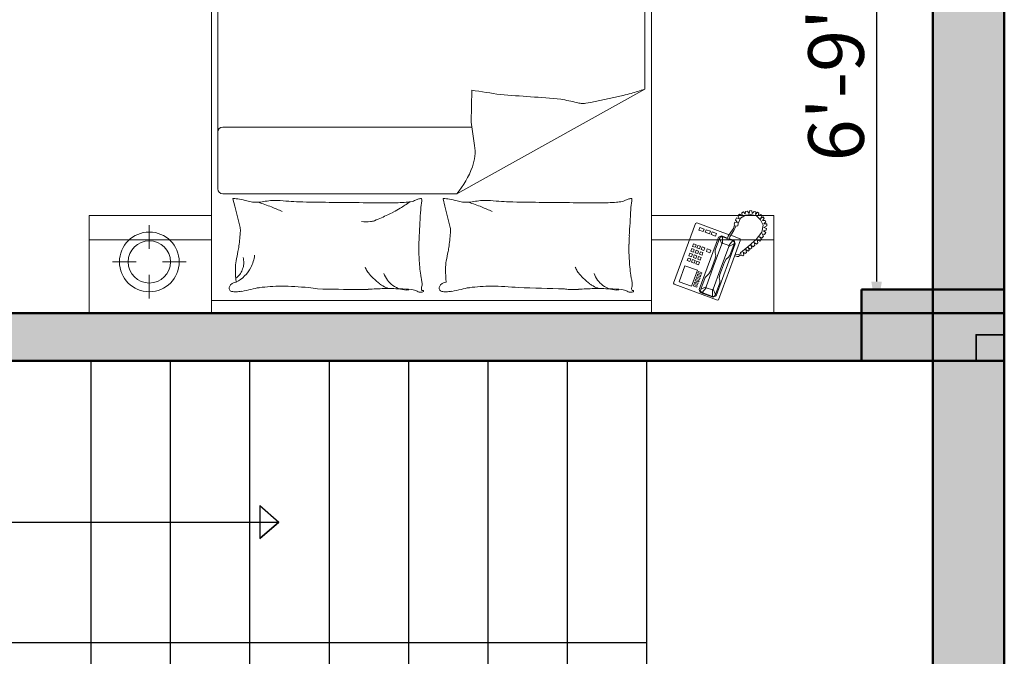
# Model space of a CAD drawing. Units: inches. Extents: x -7 to 1228, y -146 to 1091.
# Tile 83 of 88: x 1003 to 1127, y 531 to 611. Entities that reach past the tile are written whole.
import ezdxf

# ---------------------------------------------------------------- set-up
doc = ezdxf.new("R2010")
doc.units = ezdxf.units.IN
for name, color, linetype, lineweight in [('A-ANNO-DIMS', 2, 'Continuous', 18), ('A-COLS', 6, 'Continuous', 35), ('A-FLOR-STRS', 1, 'Continuous', 25), ('A-FURN', 8, 'Continuous', 18), ('A-WALL', 7, 'Continuous', 50), ('A-WALL-PATT', 251, 'Continuous', 13)]:
    doc.layers.add(name, color=color, linetype=linetype, lineweight=lineweight)
doc.styles.add('DIM_FONT', font='SIMPLEX.shx', dxfattribs={"width": 0.8})
doc.styles.get("Standard").update_dxf_attribs({"font": 'arial.ttf'})
doc.dimstyles.new('ISO-25', dxfattribs={"dimtxt": 7, "dimasz": 4, "dimexe": 1.25, "dimexo": 0.625, "dimtad": 1, "dimdec": 1, "dimlunit": 3, "dimtxsty": 'Standard', "dimcen": 2.5, "dimadec": 0, "dimazin": 0, "dimtfac": 1, "dimtdec": 1, "dimtmove": 1, "dimatfit": 3, "dimfxl": 1, "dimarcsym": 0})

# ---------------------------------------------------------------- blocks, each defined once
blk = doc.blocks.new('A$C4F634EDD')
for p, q in [((0, 2.6295), (0, 2.2295)), ((0.5, 2.6295), (0, 2.6295)), ((0.5, 2.6295), (2.3, 2.6295)), ((0.5, 0.5295), (0.5, 2.6295)), ((0.5, 2.2295), (0.5, 2.6295)), ((2.3, 2.6295), (2.3, 0.5295)), ((2.3, 2.6295), (2.8, 2.6295)), ((2.3, 2.2295), (2.3, 2.6295)), ((2.8, 2.6295), (2.8, 2.2295)), ((0.2457, 2.5697), (0.2457, 2.4733)), ((0.5, 2.5771), (2.3, 2.5771)), ((2.392, 2.5115), (2.5692, 2.5765)), ((2.4946, 2.5331), (2.4985, 2.5445)), ((2.4985, 2.5445), (2.5516, 2.564)), ((2.5062, 2.5454), (2.5004, 2.5392)), ((2.5004, 2.5392), (2.5013, 2.5315)), ((2.5062, 2.5454), (2.5487, 2.561)), ((2.5235, 2.5256), (2.5062, 2.5454)), ((2.5483, 2.5347), (2.5487, 2.561)), ((2.5487, 2.561), (2.5571, 2.56)), ((2.5615, 2.5536), (2.5514, 2.5318)), ((2.5516, 2.564), (2.5637, 2.5584)), ((2.5571, 2.56), (2.5615, 2.5536)), ((2.5615, 2.5536), (2.5791, 2.5058)), ((2.5637, 2.5584), (2.6418, 2.3458)), ((2.5692, 2.5765), (2.574, 2.5743)), ((2.574, 2.5743), (2.6638, 2.3298)), ((2.3898, 2.5066), (2.392, 2.5115)), ((2.4795, 2.2621), (2.3898, 2.5066)), ((2.412, 2.5007), (2.4634, 2.5196)), ((2.4361, 2.4352), (2.412, 2.5007)), ((2.4634, 2.5196), (2.4875, 2.454)), ((2.4842, 2.5232), (2.47, 2.518)), ((2.47, 2.518), (2.472, 2.5127)), ((2.472, 2.5127), (2.4862, 2.5179)), ((2.4881, 2.5126), (2.4739, 2.5074)), ((2.4739, 2.5074), (2.4759, 2.502)), ((2.4759, 2.502), (2.4901, 2.5073)), ((2.492, 2.5019), (2.4778, 2.4967)), ((2.4778, 2.4967), (2.4798, 2.4914)), ((2.4862, 2.5179), (2.4842, 2.5232)), ((2.4901, 2.5073), (2.4881, 2.5126)), ((2.494, 2.4966), (2.492, 2.5019)), ((2.5734, 2.3187), (2.4946, 2.5331)), ((2.5013, 2.5315), (2.5188, 2.4836)), ((2.5013, 2.5315), (2.5231, 2.5214)), ((2.5231, 2.5214), (2.5235, 2.5256)), ((2.5523, 2.4417), (2.5231, 2.5214)), ((2.5483, 2.5347), (2.5235, 2.5256)), ((2.5514, 2.5318), (2.5483, 2.5347)), ((2.5807, 2.4521), (2.5514, 2.5318)), ((2.5791, 2.5058), (2.5788, 2.4956)), ((2.4798, 2.4914), (2.494, 2.4966)), ((2.4959, 2.4913), (2.4817, 2.4861)), ((2.4817, 2.4861), (2.4837, 2.4808)), ((2.4837, 2.4808), (2.4979, 2.486)), ((2.4998, 2.4807), (2.4856, 2.4755)), ((2.4856, 2.4755), (2.4876, 2.4702)), ((2.4876, 2.4702), (2.5018, 2.4754)), ((2.5037, 2.47), (2.4895, 2.4648)), ((2.4895, 2.4648), (2.4915, 2.4595)), ((2.4915, 2.4595), (2.5057, 2.4647)), ((2.4979, 2.486), (2.4959, 2.4913)), ((2.5018, 2.4754), (2.4998, 2.4807)), ((2.5057, 2.4647), (2.5037, 2.47)), ((2.5188, 2.4836), (2.5256, 2.4761)), ((2.5256, 2.4761), (2.5342, 2.4692)), ((2.5342, 2.4692), (2.5405, 2.4574)), ((2.5405, 2.4574), (2.547, 2.4397)), ((2.5788, 2.4956), (2.5767, 2.4848)), ((2.5767, 2.4848), (2.5795, 2.4717)), ((2.5795, 2.4717), (2.586, 2.454)), ((0.0957, 2.4197), (0.192, 2.4197)), ((0.2994, 2.4197), (0.3957, 2.4197)), ((2.4875, 2.454), (2.4361, 2.4352)), ((2.4457, 2.4146), (2.4563, 2.4185)), ((2.4563, 2.4185), (2.4602, 2.4078)), ((2.4634, 2.4211), (2.474, 2.425)), ((2.4673, 2.4104), (2.4634, 2.4211)), ((2.474, 2.425), (2.4779, 2.4143)), ((2.4811, 2.4276), (2.4917, 2.4315)), ((2.485, 2.4169), (2.4811, 2.4276)), ((2.4956, 2.4208), (2.485, 2.4169)), ((2.4917, 2.4315), (2.4956, 2.4208)), ((2.5594, 2.4061), (2.547, 2.4397)), ((2.5523, 2.4417), (2.5875, 2.346)), ((2.5807, 2.4521), (2.6158, 2.3564)), ((2.5984, 2.4204), (2.586, 2.454)), ((2.6047, 2.4086), (2.5984, 2.4204)), ((2.4496, 2.4039), (2.4457, 2.4146)), ((2.4602, 2.4078), (2.4496, 2.4039)), ((2.4528, 2.3951), (2.4635, 2.399)), ((2.4567, 2.3844), (2.4528, 2.3951)), ((2.4674, 2.3883), (2.4567, 2.3844)), ((2.46, 2.3756), (2.4706, 2.3795)), ((2.4635, 2.399), (2.4674, 2.3883)), ((2.4779, 2.4143), (2.4673, 2.4104)), ((2.4706, 2.4016), (2.4812, 2.4055)), ((2.4745, 2.3909), (2.4706, 2.4016)), ((2.4706, 2.3795), (2.4745, 2.3689)), ((2.4851, 2.3949), (2.4745, 2.3909)), ((2.4777, 2.3821), (2.4883, 2.386)), ((2.4816, 2.3715), (2.4777, 2.3821)), ((2.4812, 2.4055), (2.4851, 2.3949)), ((2.4883, 2.4081), (2.4989, 2.412)), ((2.4922, 2.3975), (2.4883, 2.4081)), ((2.4883, 2.386), (2.4922, 2.3754)), ((2.5028, 2.4014), (2.4922, 2.3975)), ((2.4954, 2.3886), (2.5061, 2.3925)), ((2.4993, 2.378), (2.4954, 2.3886)), ((2.4989, 2.412), (2.5028, 2.4014)), ((2.51, 2.3819), (2.4993, 2.378)), ((2.5061, 2.3925), (2.51, 2.3819)), ((2.5238, 2.3769), (2.538, 2.3821)), ((2.5277, 2.3663), (2.5238, 2.3769)), ((2.538, 2.3821), (2.5419, 2.3715)), ((2.5622, 2.393), (2.5594, 2.4061)), ((2.5598, 2.372), (2.5601, 2.3822)), ((2.5601, 2.3822), (2.5622, 2.393)), ((2.6133, 2.4017), (2.6047, 2.4086)), ((2.6201, 2.3941), (2.6133, 2.4017)), ((2.6376, 2.3463), (2.6201, 2.3941)), ((2.6499, 2.3979), (2.6397, 2.3953)), ((2.6417, 2.39), (2.6488, 2.391)), ((2.6488, 2.391), (2.6538, 2.3895)), ((2.6551, 2.397), (2.6499, 2.3979)), ((2.6538, 2.3895), (2.6596, 2.388)), ((2.6627, 2.392), (2.6551, 2.397)), ((2.6596, 2.388), (2.6626, 2.3867)), ((2.6626, 2.3867), (2.6662, 2.388)), ((2.6692, 2.394), (2.6627, 2.392)), ((2.6662, 2.388), (2.6632, 2.3828)), ((2.6632, 2.3828), (2.6736, 2.3744)), ((2.6736, 2.3944), (2.6692, 2.394)), ((2.6765, 2.391), (2.6736, 2.3944)), ((2.6742, 2.3795), (2.6765, 2.391)), ((2.6824, 2.3858), (2.6742, 2.3795)), ((2.6873, 2.3815), (2.6824, 2.3858)), ((2.6853, 2.369), (2.6873, 2.3815)), ((2.6946, 2.376), (2.6853, 2.369)), ((2.6995, 2.3713), (2.6946, 2.376)), ((0.2457, 2.366), (0.2457, 2.2697)), ((2.4639, 2.365), (2.46, 2.3756)), ((2.4745, 2.3689), (2.4639, 2.365)), ((2.4672, 2.3561), (2.4778, 2.36)), ((2.4711, 2.3455), (2.4672, 2.3561)), ((2.4817, 2.3494), (2.4711, 2.3455)), ((2.4778, 2.36), (2.4817, 2.3494)), ((2.4922, 2.3754), (2.4816, 2.3715)), ((2.4849, 2.3626), (2.4955, 2.3665)), ((2.4888, 2.352), (2.4849, 2.3626)), ((2.4994, 2.3559), (2.4888, 2.352)), ((2.4955, 2.3665), (2.4994, 2.3559)), ((2.5026, 2.3691), (2.5132, 2.373)), ((2.5065, 2.3585), (2.5026, 2.3691)), ((2.5171, 2.3624), (2.5065, 2.3585)), ((2.5132, 2.373), (2.5171, 2.3624)), ((2.5419, 2.3715), (2.5277, 2.3663)), ((2.5774, 2.3242), (2.5598, 2.372)), ((2.5774, 2.3242), (2.5875, 2.346)), ((2.5875, 2.346), (2.5905, 2.3431)), ((2.5905, 2.3431), (2.5901, 2.3168)), ((2.6154, 2.3522), (2.5905, 2.3431)), ((2.6158, 2.3564), (2.6154, 2.3522)), ((2.6154, 2.3522), (2.6327, 2.3324)), ((2.6376, 2.3463), (2.6158, 2.3564)), ((2.6327, 2.3324), (2.6385, 2.3386)), ((2.6418, 2.3458), (2.6369, 2.332)), ((2.6385, 2.3386), (2.6376, 2.3463)), ((2.6736, 2.3744), (2.6922, 2.3593)), ((2.6922, 2.3593), (2.7051, 2.3473)), ((2.695, 2.3603), (2.6995, 2.3713)), ((2.7031, 2.3682), (2.695, 2.3603)), ((2.7096, 2.3616), (2.7031, 2.3682)), ((2.7051, 2.3473), (2.7079, 2.3475)), ((2.7062, 2.351), (2.7096, 2.3616)), ((2.7147, 2.3578), (2.7062, 2.351)), ((2.7079, 2.3475), (2.7079, 2.3443)), ((2.7079, 2.3443), (2.727, 2.3277)), ((2.7214, 2.3517), (2.7147, 2.3578)), ((2.7196, 2.34), (2.7214, 2.3517)), ((2.7286, 2.3466), (2.7196, 2.34)), ((2.7346, 2.3423), (2.7286, 2.3466)), ((2.732, 2.3295), (2.7346, 2.3423)), ((0, 2.3301), (0.5, 2.3301)), ((2.8, 2.3301), (2.3, 2.3301)), ((2.6172, 2.3086), (2.4844, 2.2599)), ((2.5114, 2.2959), (2.4936, 2.2894)), ((2.5153, 2.2853), (2.5114, 2.2959)), ((2.5362, 2.305), (2.5185, 2.2985)), ((2.5185, 2.2985), (2.5224, 2.2879)), ((2.5401, 2.2944), (2.5362, 2.305)), ((2.561, 2.3141), (2.5433, 2.3076)), ((2.5433, 2.3076), (2.5472, 2.297)), ((2.5472, 2.297), (2.5649, 2.3035)), ((2.5649, 2.3035), (2.561, 2.3141)), ((2.5855, 2.3131), (2.5734, 2.3187)), ((2.5818, 2.3178), (2.5774, 2.3242)), ((2.5901, 2.3168), (2.5818, 2.3178)), ((2.6104, 2.3222), (2.5855, 2.3131)), ((2.5901, 2.3168), (2.6097, 2.324)), ((2.613, 2.3312), (2.6077, 2.3293)), ((2.6077, 2.3293), (2.6135, 2.3141)), ((2.6192, 2.3174), (2.613, 2.3312)), ((2.6135, 2.3141), (2.6244, 2.2977)), ((2.6153, 2.3261), (2.6327, 2.3324)), ((2.6369, 2.332), (2.6161, 2.3243)), ((2.626, 2.3069), (2.6192, 2.3174)), ((2.6616, 2.3249), (2.6234, 2.3109)), ((2.6244, 2.2977), (2.6349, 2.2825)), ((2.6365, 2.2916), (2.626, 2.3069)), ((2.6638, 2.3298), (2.6616, 2.3249)), ((2.727, 2.3277), (2.7512, 2.2983)), ((2.7423, 2.3345), (2.732, 2.3295)), ((2.7406, 2.3172), (2.7495, 2.325)), ((2.7519, 2.3218), (2.7406, 2.3172)), ((2.7495, 2.325), (2.7423, 2.3345)), ((2.7512, 2.2983), (2.756, 2.2695)), ((2.7575, 2.3144), (2.7519, 2.3218)), ((2.7526, 2.3045), (2.7575, 2.3144)), ((2.7622, 2.308), (2.7526, 2.3045)), ((2.7574, 2.2924), (2.7673, 2.2997)), ((2.7673, 2.2997), (2.7622, 2.308)), ((0.5953, 2.1912), (0.616, 2.2738)), ((1.4546, 2.1912), (1.4752, 2.2738)), ((2.4844, 2.2599), (2.4795, 2.2621)), ((2.4936, 2.2894), (2.4976, 2.2788)), ((2.4976, 2.2788), (2.5153, 2.2853)), ((2.5224, 2.2879), (2.5401, 2.2944)), ((2.6349, 2.2825), (2.638, 2.273)), ((2.6407, 2.2834), (2.6365, 2.2916)), ((2.6399, 2.2712), (2.6374, 2.2659)), ((2.6374, 2.2659), (2.6398, 2.257)), ((2.638, 2.273), (2.6399, 2.2712)), ((2.6398, 2.257), (2.6509, 2.259)), ((2.6438, 2.2739), (2.6407, 2.2834)), ((2.6509, 2.259), (2.6431, 2.2492)), ((2.6519, 2.2716), (2.6438, 2.2739)), ((2.6535, 2.2628), (2.6519, 2.2716)), ((2.6636, 2.2409), (2.6535, 2.2628)), ((2.756, 2.2695), (2.7459, 2.2483)), ((2.7687, 2.2905), (2.7574, 2.2924)), ((2.7587, 2.279), (2.7699, 2.2828)), ((2.7708, 2.2725), (2.7587, 2.279)), ((2.759, 2.2637), (2.7706, 2.2643)), ((2.7676, 2.2559), (2.759, 2.2637)), ((2.7645, 2.2498), (2.7676, 2.2559)), ((2.7699, 2.2828), (2.7687, 2.2905)), ((2.7706, 2.2643), (2.7708, 2.2725)), ((0, 2.2295), (0.5, 2.2295)), ((2.8, 2.2295), (2.3, 2.2295)), ((2.6431, 2.2492), (2.6473, 2.2398)), ((2.6473, 2.2398), (2.6592, 2.2429)), ((2.6592, 2.2429), (2.6521, 2.2314)), ((2.6521, 2.2314), (2.6598, 2.2248)), ((2.6598, 2.2248), (2.6697, 2.2309)), ((2.6836, 2.2287), (2.6636, 2.2409)), ((2.6697, 2.2309), (2.6684, 2.219)), ((2.6684, 2.219), (2.6761, 2.2145)), ((2.6761, 2.2145), (2.6821, 2.2237)), ((2.6821, 2.2237), (2.6843, 2.2135)), ((2.7063, 2.2256), (2.6836, 2.2287)), ((2.6927, 2.2117), (2.6986, 2.222)), ((2.6986, 2.222), (2.7019, 2.2098)), ((2.7284, 2.2317), (2.7063, 2.2256)), ((2.7102, 2.2104), (2.7113, 2.2218)), ((2.7113, 2.2218), (2.7192, 2.2137)), ((2.7192, 2.2137), (2.7255, 2.2152)), ((2.7255, 2.2152), (2.7242, 2.2265)), ((2.7242, 2.2265), (2.7324, 2.2165)), ((2.7459, 2.2483), (2.7284, 2.2317)), ((2.7324, 2.2165), (2.7386, 2.2208)), ((2.7386, 2.2208), (2.7354, 2.2306)), ((2.7354, 2.2306), (2.7462, 2.2264)), ((2.7509, 2.2314), (2.7459, 2.2418)), ((2.7459, 2.2418), (2.7568, 2.2352)), ((2.7462, 2.2264), (2.7509, 2.2314)), ((2.7529, 2.2505), (2.7645, 2.2498)), ((2.7607, 2.2424), (2.7529, 2.2505)), ((2.7568, 2.2352), (2.7607, 2.2424)), ((0.5878, 2.1612), (0.5953, 2.1912)), ((1.4471, 2.1612), (1.4546, 2.1912)), ((2.6843, 2.2135), (2.6927, 2.2117)), ((2.7019, 2.2098), (2.7102, 2.2104)), ((1.5035, 2.141), (0.5458, 2.141)), ((1.5035, 2.141), (2.2716, 1.7136)), ((0.5258, 2.121), (0.5258, 0.5617)), ((1.576, 1.9433), (1.5624, 1.8479)), ((0.5458, 1.8684), (1.5653, 1.8684)), ((1.5624, 1.8479), (1.5641, 1.7178)), ((2.2716, 0.5617), (2.2716, 1.7136))]:
    blk.add_line(p, q)
for radius in [0.1222, 0.0865]:
    blk.add_circle((0.2457, 2.4197), radius)
for centre, radius, start, end in [((0.5848, 2.5274), 0.0131, 101.2724, 206.5805), ((0.5999, 2.4516), 0.0904, 90, 101.2724), ((0.5999, 2.3808), 0.1611, 81.5628, 90), ((0.5788, 2.2388), 0.3048, 74.256, 81.5628), ((1.3132, 2.5864), 0.0539, 275.2592, 300.6513), ((1.3554, 2.5152), 0.0289, 85.6975, 120.6513), ((1.3556, 2.519), 0.0251, 68.2117, 85.6975), ((1.3634, 2.533), 0.00428, 78.1069, 158.0096), ((1.3647, 2.5395), 0.00232, 258.1069, 19.564), ((1.3637, 2.5391), 0.00342, 19.564, 68.2117), ((1.444, 2.5274), 0.0131, 101.2724, 206.5805), ((1.4591, 2.4516), 0.0904, 90, 101.2724), ((1.4591, 2.3808), 0.1611, 81.5628, 90), ((1.438, 2.2388), 0.3048, 74.256, 81.5628), ((2.1724, 2.5864), 0.0539, 275.2592, 300.6513), ((2.2146, 2.5152), 0.0289, 85.6975, 120.6513), ((2.2149, 2.519), 0.0251, 68.2117, 85.6975), ((2.2226, 2.533), 0.00428, 78.1069, 158.0096), ((2.224, 2.5395), 0.00232, 258.1069, 19.564), ((2.2229, 2.5391), 0.00342, 19.564, 68.2117), ((0.6036, 2.5368), 0.0342, 206.5805, 265.5998), ((1.0898, 2.4496), 0.4918, 173.7676, 180), ((0.5368, 2.3783), 0.1399, 45.0976, 62.7964), ((0.7272, 2.7653), 0.2422, 254.256, 262.4531), ((0.7851, 3.2019), 0.6827, 262.4531, 270), ((0.7851, 3.5682), 1.049, 270, 276.0867), ((0.8402, 3.0514), 0.5293, 276.0867, 280.1899), ((1.1602, -8.1346), 10.6675, 90.30153, 91.21582), ((1.1169, 2.2433), 0.2897, 85.1982, 92.5386), ((1.2142, 3.4021), 0.8732, 265.1982, 269.4243), ((1.4317, 2.2032), 0.3916, 128.3886, 133.8115), ((1.2362, 2.45), 0.0768, 117.2396, 128.3886), ((1.3082, 2.3102), 0.234, 110.8603, 117.2396), ((1.2204, 4.0232), 1.4943, 269.4243, 271.9079), ((1.2995, 2.4357), 0.0992, 126.0864, 143.8234), ((1.2995, 2.4357), 0.0992, 105.9352, 126.0864), ((1.2429, 3.3501), 0.8208, 271.9079, 275.2592), ((1.2995, 2.4357), 0.0992, 85.7841, 105.9352), ((1.3739, 2.5288), 0.0156, 158.0096, 201.421), ((1.1177, 2.5413), 0.246, 347.8905, 351.8665), ((1.3288, 2.5111), 0.0328, 351.8665, 21.421), ((1.4628, 2.5368), 0.0342, 206.5805, 265.5998), ((1.949, 2.4496), 0.4918, 173.7676, 180), ((1.5865, 2.7653), 0.2422, 254.256, 262.4531), ((1.6443, 3.2019), 0.6827, 262.4531, 270), ((1.6443, 3.5682), 1.049, 270, 276.0867), ((1.4785, 15.4878), 12.9656, 271.22425, 272.05324), ((1.97, 2.3805), 0.1524, 92.5386, 100.1899), ((1.9761, 2.2433), 0.2897, 85.1982, 92.5386), ((2.0734, 3.4021), 0.8732, 265.1982, 269.4243), ((2.291, 2.2032), 0.3916, 128.3886, 133.8115), ((2.0954, 2.45), 0.0768, 117.2396, 128.3886), ((2.1674, 2.3102), 0.234, 110.8603, 117.2396), ((2.0797, 4.0232), 1.4943, 269.4243, 271.9079), ((2.1588, 2.4357), 0.0992, 126.0864, 143.8234), ((2.1588, 2.4357), 0.0992, 105.9352, 126.0864), ((2.1021, 3.3501), 0.8208, 271.9079, 275.2592), ((2.1588, 2.4357), 0.0992, 85.7841, 105.9352), ((2.2331, 2.5288), 0.0156, 158.0096, 201.421), ((1.977, 2.5413), 0.246, 347.8905, 351.8665), ((2.1881, 2.5111), 0.0328, 351.8665, 21.421), ((0.5462, 2.4142), 0.0899, 41.4429, 53.7359), ((0.5741, 2.4389), 0.0526, 25.3551, 41.4429), ((0.4851, 2.3967), 0.1511, 21.8149, 25.3551), ((0.5368, 2.3783), 0.1399, 27.3988, 45.0976), ((1.3127, 2.3625), 0.2002, 151.6832, 156.9972), ((1.1799, 2.4341), 0.0493, 140.9651, 151.6832), ((1.3165, 2.3233), 0.2252, 133.8115, 140.9651), ((1.2995, 2.4357), 0.0992, 143.8234, 161.5603), ((2.2605, 2.3525), 0.9131, 172.3191, 176.6313), ((1.5522, 2.448), 0.1983, 167.8905, 172.3191), ((2.1719, 2.3625), 0.2002, 151.6832, 156.9972), ((2.0391, 2.4341), 0.0493, 140.9651, 151.6832), ((2.1757, 2.3233), 0.2252, 133.8115, 140.9651), ((2.1588, 2.4357), 0.0992, 143.8234, 161.5603), ((3.1198, 2.3525), 0.9131, 172.3191, 176.6313), ((2.4114, 2.448), 0.1983, 167.8905, 172.3191), ((0.8019, 2.4496), 0.204, 180, 189.6844), ((0.4345, 2.3765), 0.2056, 18.7799, 21.8149), ((0.576, 2.4246), 0.0562, 0, 18.7799), ((0.5406, 2.4246), 0.0915, 345.3149, 0), ((0.5368, 2.3783), 0.1399, 16.515, 27.3988), ((0.5368, 2.3783), 0.1399, 5.6311, 16.515), ((1.6611, 2.4496), 0.204, 180, 189.6844), ((1.4703, 2.5637), 0.882, 189.6844, 192.1984), ((0.2982, 2.3103), 0.3171, 8.0051, 12.1984), ((2.0266, 2.3663), 0.6787, 176.6313, 181.6331), ((2.3295, 2.5637), 0.882, 189.6844, 192.1984), ((1.1575, 2.3103), 0.3171, 8.0051, 12.1984), ((2.8858, 2.3663), 0.6787, 176.6313, 181.6331), ((-0.0401, 2.2627), 0.6588, 2.6649, 8.0051), ((2.7128, 2.3859), 1.3652, 181.6331, 183.055), ((0.8191, 2.2627), 0.6588, 2.6649, 8.0051), ((3.5721, 2.3859), 1.3652, 181.6331, 183.055), ((14.9657, 3.0398), 13.6356, 183.05496, 183.50486), ((15.8249, 3.0398), 13.6356, 183.05496, 183.50486), ((0.5503, 2.2902), 0.0677, 345.9548, 2.6649), ((1.1303, 1.9835), 0.2721, 85.9172, 93.5552), ((1.4096, 2.2902), 0.0677, 345.9548, 2.6649), ((1.1455, 2.197), 0.058, 69.3257, 85.9172), ((0.9871, 1.7772), 0.5066, 65.6735, 69.3257), ((0.6058, 0.9338), 1.4323, 63.5015, 65.6735), ((1.1054, 1.9358), 0.3126, 57.865, 63.5015), ((0.6807, 2.0561), 0.1197, 96.4341, 107.3864), ((0.6836, 2.0301), 0.1459, 78.4414, 96.4341), ((0.473, 2.8815), 0.7387, 287.1982, 289.428), ((0.473, 2.8815), 0.7387, 289.428, 291.6577), ((0.473, 2.8815), 0.7387, 291.6577, 293.4844), ((0.473, 2.8815), 0.7387, 293.4844, 295.3111), ((1.2501, -19.8405), 22.0183, 90.37908, 91.01965), ((1.2012, -3.5404), 5.7185, 89.7135, 90.9704), ((1.224, 1.0141), 1.164, 86.426, 89.7135), ((0.8841, 1.5835), 0.7286, 54.1737, 57.865), ((1.2875, 2.0302), 0.1459, 77.131, 86.426), ((1.6762, 2.2258), 0.3212, 183.5049, 189.9984), ((1.5399, 2.0561), 0.1197, 96.4341, 107.3864), ((1.5429, 2.0301), 0.1459, 78.4414, 96.4341), ((1.3322, 2.8815), 0.7387, 287.1982, 289.428), ((1.3322, 2.8815), 0.7387, 289.428, 291.6577), ((1.3322, 2.8815), 0.7387, 291.6577, 293.4844), ((1.3322, 2.8815), 0.7387, 293.4844, 295.3111), ((2.1093, -19.8405), 22.0183, 90.37908, 91.01965), ((2.0605, -3.5404), 5.7185, 89.7135, 90.9704), ((2.0833, 1.0141), 1.164, 86.426, 89.7135), ((2.1467, 2.0302), 0.1459, 77.131, 86.426), ((2.5355, 2.2258), 0.3212, 183.5049, 189.9984), ((0.5458, 2.121), 0.02, 90, 180), ((0.5887, 2.1609), 0.000917, 165.9551, 274.0829), ((0.5695, 2.4301), 0.2708, 274.0829, 279.4841), ((0.5763, 2.3896), 0.2297, 279.4841, 287.3864), ((0.759, 2.3985), 0.2301, 258.4414, 272.7491), ((0.7026, 3.5718), 1.4048, 272.7491, 274.6176), ((0.9136, 0.9591), 1.2165, 92.6096, 94.6176), ((1.3099, 2.1283), 0.0453, 62.7159, 77.131), ((1.3658, 2.2367), 0.0767, 242.7159, 253.7788), ((1.3688, 2.247), 0.0875, 253.7788, 262.8796), ((1.3581, 2.1615), 0.00132, 262.8796, 343.3022), ((1.3409, 2.1667), 0.0193, 343.3022, 9.9984), ((1.448, 2.1609), 0.000917, 165.9551, 274.0829), ((1.4288, 2.4301), 0.2708, 274.0829, 279.4841), ((1.4355, 2.3896), 0.2297, 279.4841, 287.3864), ((1.2147, 1.9017), 0.3751, 20.1488, 39.6445), ((1.6182, 2.3985), 0.2301, 258.4414, 272.7491), ((1.5619, 3.5718), 1.4048, 272.7491, 274.6176), ((1.7729, 0.9591), 1.2165, 92.6096, 94.6176), ((2.1691, 2.1283), 0.0453, 62.7159, 77.131), ((2.2251, 2.2367), 0.0767, 242.7159, 253.7788), ((2.2281, 2.247), 0.0875, 253.7788, 262.8796), ((2.2174, 2.1615), 0.00132, 262.8796, 343.3022), ((2.2001, 2.1667), 0.0193, 343.3022, 9.9984), ((1.3977, 1.9688), 0.1801, 351.8644, 20.1488), ((0.5458, 1.8884), 0.02, 180, 270), ((2.0195, 1.7137), 0.0581, 79.2724, 97.7304), ((1.0582, 5.4638), 3.7801, 277.692, 279.495), ((0.6102, 18.0525), 16.3521, 273.75703, 274.62393), ((1.4194, 4.2174), 2.5158, 281.6741, 283.1904), ((2.0378, 1.5789), 0.1942, 97.7304, 103.1904), ((1.2737, -2.2227), 4.0646, 77.0745, 79.2724), ((2.0359, 1.0981), 0.6574, 74.0648, 77.0745), ((1.7125, -0.0344), 1.8351, 72.2636, 74.0648)]:
    blk.add_arc(centre, radius, start, end)
at = {"style": 'DIM_FONT', "width": 0.8, "flags": 9}
for tag, p in [('YSIZE', (0.5, 2.6295)), ('XSIZE', (0.5, 2.6295)), ('XSIZE', (2.2985, 2.6295)), ('YSIZE', (2.2985, 2.6295))]:
    blk.add_attdef(tag, p, '', height=0.0005, dxfattribs=at)
blk = doc.blocks.new('*D27')
at = {"layer": 'A-ANNO-DIMS', "color": 0, "lineweight": -2, "transparency": 16777216}
for p, q in [((1098.61, 654.97), (1112.17, 654.97)), ((1110.92, 650.97), (1110.92, 577.98)), ((1098.61, 573.98), (1112.17, 573.98))]:
    blk.add_line(p, q, dxfattribs=at)
at = {"layer": 'A-ANNO-DIMS', "color": 0, "transparency": 16777216}
for points in [[(1110.25, 650.97), (1111.58, 650.97), (1110.92, 654.97)], [(1110.25, 577.98), (1111.58, 577.98), (1110.92, 573.98)]]:
    blk.add_solid(points, dxfattribs=at)
at = {"layer": 'Defpoints', "color": 0, "transparency": 16777216}
for p in [(1097.98, 654.97), (1097.98, 573.98), (1110.92, 573.98)]:
    blk.add_point(p, dxfattribs=at)
at = {"layer": 'A-ANNO-DIMS', "color": 0, "transparency": 16777216, "insert": (1106.72, 614.48), "char_height": 7, "attachment_point": 5, "rotation": 90}
blk.add_mtext('6\'-9" TYP.', dxfattribs=at)

msp = doc.modelspace()

# ---------------------------------------------------------------- hatches: boundary and pattern name
at = {"layer": 'A-COLS'}
h = msp.add_hatch(color=256, dxfattribs=at)
h.dxf.hatch_style = 1
h.paths.add_polyline_path([(1123.45, 568), (1123.45, 571.29), (1127, 571.29), (1127, 577), (1109, 577), (1109, 568)])
h = msp.add_hatch(color=256, dxfattribs=at)
h.dxf.hatch_style = 1
h.paths.add_polyline_path([(1123.45, 568), (1127, 568), (1127, 571.29), (1123.45, 571.29)])
at = {"layer": 'A-WALL-PATT'}
h = msp.add_hatch(color=256, dxfattribs=at)
h.dxf.hatch_style = 1
h.paths.add_polyline_path([(69, 568), (60, 568), (60, 493), (63.29, 493), (69, 493)])
h.paths.add_polyline_path([(69, 662.41), (60, 662.41), (60, 586), (69, 586)], flags=17)
h.paths.add_polyline_path([(69, 723), (184, 723), (184, 734), (179, 734), (179, 728), (69, 728), (69, 741.62), (60, 741.62), (60, 698.41), (69, 698.41)], flags=17)
h.paths.add_polyline_path([(69, 782), (231, 782), (231, 728), (231, 723), (231, 586), (236, 586), (236, 787), (69, 787), (69, 800.13), (60, 800.13), (60, 765.62), (69, 765.62)])
h.paths.add_polyline_path([(184, 842), (189, 842), (189, 848), (173, 848), (173, 842), (179, 842), (179, 787), (184, 787)])
h.paths.add_polyline_path([(118.22, 69), (69, 69), (69, 60), (118.22, 60)])
h.paths.add_polyline_path([(227, 69), (154.22, 69), (154.22, 60), (227, 60)])
h.paths.add_polyline_path([(236, 60), (232.71, 60), (227, 60), (227, 36), (236, 36)])
h.paths.add_polyline_path([(389, 60), (380, 60), (380, 36), (389, 36)])
h.paths.add_polyline_path([(384, 181), (380, 181), (380, 115), (380, 78), (384, 78)])
h.paths.add_polyline_path([(380, 115), (334.55, 115), (334.55, 109), (380, 109)])
h.paths.add_polyline_path([(274.55, 115), (236, 115), (236, 201), (232.71, 201), (231, 201), (231, 78), (236, 78), (236, 109), (274.55, 109)])
h.paths.add_polyline_path([(69, 123), (60, 123), (60, 78), (69, 78)])
h.paths.add_polyline_path([(69, 201), (60, 201), (60, 159), (69, 159)])
h.paths.add_polyline_path([(143, 219), (69, 219), (69, 213), (143, 213)], flags=17)
h.paths.add_polyline_path([(189, 219), (184, 219), (184, 274), (231, 274), (231, 219), (236, 219), (236, 279), (184, 279), (184, 297), (179, 297), (179, 279), (69, 279), (69, 290.91), (60, 290.91), (60, 262.18), (69, 262.18), (69, 274), (179, 274), (179, 219), (173, 219), (173, 213), (189, 213)])
h.paths.add_polyline_path([(69, 238.18), (60, 238.18), (60, 219), (69, 219)], flags=17)
h.paths.add_polyline_path([(69, 333), (60, 333), (60, 314.91), (69, 314.91), (69, 316.96)])
h.paths.add_polyline_path([(190, 338), (184, 338), (69, 338), (69, 333), (179, 333), (179, 327), (184, 327), (184, 333.02), (190, 333.05)])
h.paths.add_polyline_path([(69, 386.81), (60, 386.81), (60, 351), (69, 351)])
h.paths.add_polyline_path([(69, 475), (60, 475), (60, 422.81), (69, 422.81)])
h.paths.add_polyline_path([(236, 475), (231, 475), (231, 351.24), (236, 351.24)])
h.paths.add_polyline_path([(384, 475), (380, 475), (380, 362), (384, 362)])
h.paths.add_polyline_path([(547, 307), (439, 307), (439, 356), (445, 356), (445, 362), (433, 362), (433, 307), (380, 307), (380, 244), (380, 241), (384, 241), (384, 301), (433, 301), (433, 277), (439, 277), (439, 301), (547, 301)])
h.paths.add_polyline_path([(547, 241), (439, 241), (439, 247), (433, 247), (433, 235), (547, 235)])
h.paths.add_polyline_path([(450, 69), (440.29, 69), (424.89, 69), (389, 69), (389, 60), (450, 60)])
h.paths.add_polyline_path([(547, 69), (486, 69), (486, 60), (547, 60)])
h.paths.add_polyline_path([(556, 148.27), (547, 148.27), (547, 78), (556, 78)])
h.paths.add_polyline_path([(556, 223), (547, 223), (547, 195), (547, 184.27), (556, 184.27)])
h.paths.add_polyline_path([(556, 311.19), (547, 311.19), (547, 273.08), (556, 273.08)])
h.paths.add_polyline_path([(556, 344), (552.71, 344), (547, 344), (547, 335.19), (556, 335.19)])
h.paths.add_polyline_path([(556, 249.08), (547, 249.08), (547, 241), (556, 241)])
h.paths.add_polyline_path([(547, 362), (475, 362), (475, 356), (547, 356)], flags=0)
h.paths.add_polyline_path([(556, 399.62), (547, 399.62), (547, 362), (556, 362)])
h.paths.add_polyline_path([(556, 475), (547, 475), (547, 435.62), (556, 435.62)])
h.paths.add_polyline_path([(547, 493), (389, 493), (389, 487), (547, 487)])
h.paths.add_polyline_path([(380, 493), (278, 493), (278, 487), (380, 487)])
h.paths.add_polyline_path([(227, 493), (69, 493), (69, 487), (227, 487)])
h.paths.add_polyline_path([(643, 122.44), (634, 122.44), (634, 78), (643, 78)])
h.paths.add_polyline_path([(702.5, 69), (692.79, 69), (677.39, 69), (643, 69), (643, 60), (702.5, 60)])
h.paths.add_polyline_path([(798, 69), (738.5, 69), (738.5, 60), (798, 60)])
h.paths.add_polyline_path([(807, 60), (803.71, 60), (798, 60), (798, 36), (807, 36)])
h.paths.add_polyline_path([(807, 109), (846.75, 109), (846.75, 115), (807, 115), (807, 159), (802, 159), (802, 78), (807, 78)])
h.paths.add_polyline_path([(807, 201), (802, 201), (802, 195), (807, 195)])
h.paths.add_polyline_path([(643, 201), (634, 201), (634, 158.44), (643, 158.44)])
h.paths.add_polyline_path([(756, 225), (751, 225), (751, 219), (643, 219), (643, 213), (756, 213)])
h.paths.add_polyline_path([(643, 240.85), (634, 240.85), (634, 219), (643, 219)])
h.paths.add_polyline_path([(643, 274), (643, 288.63), (634, 288.63), (634, 264.85), (643, 264.85)])
h.paths.add_polyline_path([(802, 279), (756, 279), (756, 297), (751, 297), (751, 279), (643, 279), (643, 274), (751, 274), (751, 255), (756, 255), (756, 274), (802, 274)])
h.paths.add_polyline_path([(807, 333), (803.71, 333), (802, 333), (802, 279), (802, 274), (802, 219), (807, 219)])
h.paths.add_polyline_path([(956, 182), (951, 182), (951, 115), (906.75, 115), (906.75, 109), (951, 109), (951, 78), (956, 78)])
h.paths.add_polyline_path([(960, 60), (951, 60), (951, 36), (960, 36)])
h.paths.add_polyline_path([(1021, 69), (1005.78, 69), (960, 69), (960, 60), (1021, 60)])
h.paths.add_polyline_path([(956, 224), (951, 224), (951, 218), (956, 218)])
h.paths.add_polyline_path([(956, 302), (1004, 302), (1004, 278), (1010, 278), (1010, 302), (1118, 302), (1118, 290.81), (1127, 290.81), (1127, 326.97), (1118, 326.97), (1118, 320.97), (1118, 307), (1010, 307), (1010, 356), (1016, 356), (1016, 362), (1004, 362), (1004, 307), (951, 307), (951, 244), (951, 242), (954.29, 242), (956, 242)])
h.paths.add_polyline_path([(643, 333), (634, 333), (634, 312.63), (643, 312.63), (643, 316.96)])
h.paths.add_polyline_path([(756, 338), (643, 338), (643, 333), (751, 333), (751, 327), (756, 327)])
h.paths.add_polyline_path([(643, 388), (634, 388), (634, 351), (643, 351)])
h.paths.add_polyline_path([(807, 357), (802, 357), (802, 351), (807, 351)])
h.paths.add_polyline_path([(807, 475), (802, 475), (802, 393), (807, 393)])
h.paths.add_polyline_path([(643, 475), (634, 475), (634, 424), (643, 424)])
h.paths.add_polyline_path([(798, 493), (643, 493), (643, 487), (798, 487)])
h.paths.add_polyline_path([(634, 493), (556, 493), (556, 487), (634, 487)])
h.paths.add_polyline_path([(813, 493), (807, 493), (807, 487), (813, 487)])
h.paths.add_polyline_path([(951, 493), (849, 493), (849, 487), (951, 487)])
h.paths.add_polyline_path([(956, 484), (951, 484), (951, 374), (956, 374)])
h.paths.add_polyline_path([(1109, 493), (969, 493), (969, 487), (1109, 487)])
h.paths.add_polyline_path([(1127, 484), (1118, 484), (1118, 450.64), (1127, 450.64)])
h.paths.add_polyline_path([(1127, 414.64), (1118, 414.64), (1118, 365), (1127, 365)])
h.paths.add_polyline_path([(1109, 362), (1046, 362), (1046, 356), (1109, 356)], flags=17)
h.paths.add_polyline_path([(1127, 356), (1123.45, 356), (1118, 356), (1118, 350.97), (1127, 350.97)], flags=0)
h.paths.add_polyline_path([(1127, 266.81), (1118, 266.81), (1118, 262.36), (1118, 242), (1127, 242)], flags=17)
h.paths.add_polyline_path([(1118, 242), (1010, 242), (1010, 248), (1004, 248), (1004, 237), (1118, 237)])
h.paths.add_polyline_path([(1127, 224), (1118, 224), (1118, 170), (1127, 170)])
h.paths.add_polyline_path([(1127, 134), (1118, 134), (1118, 78), (1127, 78)])
h.paths.add_polyline_path([(1118, 69), (1057, 69), (1057, 60), (1118, 60)])
h.paths.add_polyline_path([(227, 571.55), (227, 574), (69, 574), (69, 568), (227, 568)])
h.paths.add_polyline_path([(380, 571.55), (380, 574), (278, 574), (278, 568), (380, 568)])
h.paths.add_polyline_path([(242, 574), (236, 574), (236, 568), (242, 568)])
h.paths.add_polyline_path([(547, 571.55), (547, 574), (389, 574), (389, 568), (547, 568)])
h.paths.add_polyline_path([(384, 733), (380, 733), (380, 586), (384, 586)])
h.paths.add_polyline_path([(556, 646), (634, 646), (634, 655), (547, 655), (547, 586), (556, 586)])
h.paths.add_polyline_path([(634, 574), (556, 574), (556, 568), (634, 568)])
h.paths.add_polyline_path([(643, 655), (634, 655), (634, 586), (643, 586)])
h.paths.add_polyline_path([(798, 574), (643, 574), (643, 568), (798, 568)])
h.paths.add_polyline_path([(643, 663.85), (634, 663.85), (634, 655), (643, 655)])
h.paths.add_polyline_path([(556, 676.97), (547, 676.97), (547, 655), (556, 655)])
h.paths.add_polyline_path([(556, 733), (547, 733), (547, 712.97), (556, 712.97)])
h.paths.add_polyline_path([(643, 710), (634, 710), (634, 699.85), (643, 699.85)])
h.paths.add_polyline_path([(807, 668), (802, 668), (802, 586), (807, 586)])
h.paths.add_polyline_path([(951, 574), (849, 574), (849, 568), (951, 568)])
h.paths.add_polyline_path([(956, 691), (951, 691), (951, 577), (956, 577)])
h.paths.add_polyline_path([(1109, 574), (969, 574), (969, 568), (1109, 568)])
h.paths.add_polyline_path([(1127, 643.4), (1118, 643.4), (1118, 577), (1127, 577)])
h.paths.add_polyline_path([(1127, 568), (1123.45, 568), (1118, 568), (1118, 493), (1127, 493)])
h.paths.add_polyline_path([(1127, 733), (1118, 733), (1118, 679.4), (1127, 679.4)])
h.paths.add_polyline_path([(1127, 777.35), (1118, 777.35), (1118, 770.04), (1118, 751), (1127, 751)], flags=17)
h.paths.add_polyline_path([(1118, 751), (1010, 751), (1010, 757), (1004, 757), (1004, 745), (1118, 745)])
h.paths.add_polyline_path([(956, 811), (1004, 811), (1004, 787), (1010, 787), (1010, 811), (1017.87, 811), (1017.87, 811.63, -0.414214), (1018.25, 812), (1031.98, 812, -0.414214), (1032.35, 811.63), (1032.35, 811), (1118, 811), (1118, 801.35), (1127, 801.35), (1127, 834.69), (1118, 834.69), (1118, 830.24), (1118, 817), (1010, 817), (1010, 866), (1016, 866), (1016, 872), (1004, 872), (1004, 817), (956, 817), (956, 866), (951, 866), (951, 751), (954.29, 751), (956, 751)])
h.paths.add_polyline_path([(1118, 872), (1046, 872), (1046, 866), (1118, 866)], flags=17)
h.paths.add_polyline_path([(1127, 924.71), (1118, 924.71), (1118, 884), (1127, 884)])
h.paths.add_polyline_path([(1127, 866), (1123.71, 866), (1118, 866), (1118, 858.69), (1127, 858.69)], flags=17)
h.paths.add_polyline_path([(956, 983), (951, 983), (951, 952), (807, 952), (807, 983), (802, 983), (802, 902), (807, 902), (807, 946), (951, 946), (951, 884), (956, 884)])
h.paths.add_polyline_path([(807, 842), (802, 842), (802, 787), (756, 787), (756, 806), (751, 806), (751, 787), (643, 787), (643, 782), (751, 782), (751, 764), (756, 764), (756, 782), (802, 782), (802, 728), (807, 728)])
h.paths.add_polyline_path([(756, 848), (643, 848), (643, 842), (751, 842), (751, 836), (756, 836)])
h.paths.add_polyline_path([(756, 734), (751, 734), (751, 728), (643, 728), (643, 723), (756, 723)])
h.paths.add_polyline_path([(643, 749.79), (634, 749.79), (634, 728), (637.29, 728), (643, 728)])
h.paths.add_polyline_path([(643, 805.41), (634, 805.41), (634, 773.79), (643, 773.79)])
h.paths.add_polyline_path([(643, 896.66), (634, 896.66), (634, 860), (637.29, 860), (643, 860)])
h.paths.add_polyline_path([(643, 842), (634, 842), (634, 829.41), (643, 829.41)])
h.paths.add_polyline_path([(643, 983), (634, 983), (634, 932.66), (643, 932.66)])
h.paths.add_polyline_path([(1127, 983), (1118, 983), (1118, 960.71), (1127, 960.71)])
h.paths.add_polyline_path([(1118, 1001), (1077.53, 1001), (1077.53, 992), (1118, 992)])
h.paths.add_polyline_path([(1041.53, 1001), (960, 1001), (960, 992), (1041.53, 992)])
h.paths.add_polyline_path([(960, 1025), (951, 1025), (951, 1001), (954.29, 1001), (960, 1001)])
h.paths.add_polyline_path([(807, 1025), (798, 1025), (798, 1001), (807, 1001)])
h.paths.add_polyline_path([(798, 1001), (738.5, 1001), (738.5, 992), (798, 992)])
h.paths.add_polyline_path([(702.5, 1001), (643, 1001), (643, 992), (702.5, 992)])
h.paths.add_polyline_path([(547, 1001), (499.11, 1001), (499.11, 992), (547, 992)])
h.paths.add_polyline_path([(463.11, 1001), (389, 1001), (389, 992), (463.11, 992)])
h.paths.add_polyline_path([(389, 1025), (380, 1025), (380, 1022), (380, 1001), (383.29, 1001), (389, 1001)])
h.paths.add_polyline_path([(236, 1025), (227, 1025), (227, 1001), (236, 1001)])
h.paths.add_polyline_path([(236, 983), (231, 983), (231, 860), (236, 860)])
h.paths.add_polyline_path([(274.55, 952), (236, 952), (236, 946), (274.55, 946)])
h.paths.add_polyline_path([(380, 952), (334.55, 952), (334.55, 946), (380, 946)])
h.paths.add_polyline_path([(384, 983), (380, 983), (380, 884), (383.29, 884), (384, 884)])
h.paths.add_polyline_path([(227, 1001), (155.01, 1001), (155.01, 992), (162.87, 992), (227, 992)])
h.paths.add_polyline_path([(119.01, 1001), (69, 1001), (69, 992), (119.01, 992)])
h.paths.add_polyline_path([(69, 983), (60, 983), (60, 922.99), (69, 922.99)])
h.paths.add_polyline_path([(69, 886.99), (60, 886.99), (60, 860), (63.29, 860), (69, 860)])
h.paths.add_polyline_path([(143, 848), (69, 848), (69, 842), (143, 842)])

# ---------------------------------------------------------------- linework, layer by layer
at = {"layer": 'A-COLS'}
msp.add_lwpolyline([(1127, 568), (1127, 571.29), (1123.45, 571.29), (1123.45, 568)], close=True, dxfattribs=at)
at = {"layer": 'A-FLOR-STRS'}
for p, q in [((1012, 493), (1012, 568)), ((1022, 493), (1022, 568)), ((1032, 493), (1032, 568)), ((1042, 493), (1042, 568)), ((1052, 493), (1052, 568)), ((1062, 493), (1062, 568)), ((1072, 493), (1072, 568)), ((1082, 493), (1082, 568)), ((1033.23, 549.76), (1035.65, 547.69)), ((1033.23, 549.76), (1033.23, 545.62)), ((982.86, 547.69), (1035.65, 547.69)), ((1035.65, 547.69), (1033.23, 545.62)), ((1033.23, 545.62), (1035.65, 547.69)), ((992, 532.5), (1082, 532.5))]:
    msp.add_line(p, q, dxfattribs=at)
at = {"layer": 'A-WALL'}
for p, q in [((1127, 60), (1127, 1001)), ((1118, 307), (1118, 811)), ((1127, 577), (1109, 577)), ((1109, 577), (1109, 568)), ((1127, 568), (1127, 577)), ((1127, 574), (849, 574)), ((1127, 568), (849, 568)), ((1109, 568), (1127, 568))]:
    msp.add_line(p, q, dxfattribs=at)

# ---------------------------------------------------------------- block references
at = {"layer": 'A-FURN', "xscale": -30.79356024027943, "yscale": 30.79356024027943, "zscale": 30.79356024027943, "rotation": 180}
msp.add_blockref('A$C4F634EDD', (1011.76, 654.97), dxfattribs=at)

# ---------------------------------------------------------------- dimensions: what is measured, and where the dimension line sits
at = {"layer": 'A-ANNO-DIMS'}
dim = msp.add_linear_dim(base=(1110.92, 573.98), p1=(1097.98, 654.97), p2=(1097.98, 573.98), angle=270, text='<> TYP.', dimstyle='ISO-25', override={"dimdec": 1, "dimlfac": 1, "dimrnd": 0, "dimzin": 1, "dimdsep": 46, "dimlunit": 4, "dimfrac": 2}, dxfattribs=at)
dim.commit()
dim.dimension.update_dxf_attribs({"geometry": '*D27', "text_midpoint": (1106.72, 614.48)})

doc.saveas('drawing.dxf')
